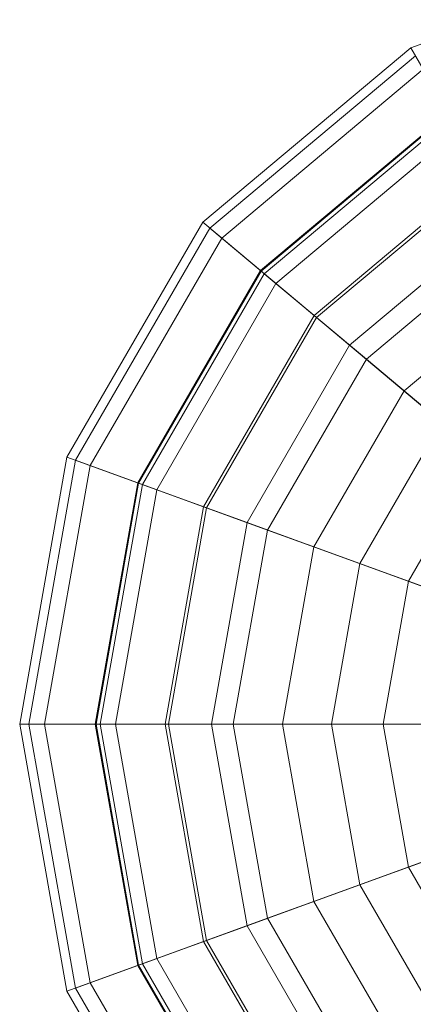
# Model space of a CAD drawing. Units: inches. Extents: x 375 to 1122, y 27 to 1069.
# Tile 31 of 155: x 731.708 to 732.389, y 280.756 to 282.464. Entities that reach past the tile are written whole.
import ezdxf

# ---------------------------------------------------------------- set-up
doc = ezdxf.new("R2010")
doc.units = ezdxf.units.IN
doc.layers.add('Furniture', color=30, linetype='Continuous', lineweight=18)

# ---------------------------------------------------------------- blocks, each defined once
blk = doc.blocks.new('A$C403C54AD')
for points in [[(1.593116, 1.197037, -0.04658), (1.626464, 1.202917, -0.043501), (1.626464, 1.202917, -0.043501), (1.597139, 1.185986, -0.04658)], [(1.597139, 1.185986, -0.04658), (1.626464, 1.202917, -0.043501), (1.626464, 1.202917, -0.043501), (1.604698, 1.176977, -0.04658)], [(1.604698, 1.176977, -0.04658), (1.626464, 1.202917, -0.043501), (1.626464, 1.202917, -0.043501), (1.614883, 1.171097, -0.04658)], [(1.614883, 1.171097, -0.04658), (1.626464, 1.202917, -0.043501), (1.626464, 1.202917, -0.043501), (1.626464, 1.169055, -0.04658)], [(1.65579, 1.185986, -0.04658), (1.626464, 1.202917, -0.043501), (1.626464, 1.202917, -0.043501), (1.659812, 1.197037, -0.04658)], [(1.64823, 1.176977, -0.04658), (1.626464, 1.202917, -0.043501), (1.626464, 1.202917, -0.043501), (1.65579, 1.185986, -0.04658)], [(1.638046, 1.171097, -0.04658), (1.626464, 1.202917, -0.043501), (1.626464, 1.202917, -0.043501), (1.64823, 1.176977, -0.04658)], [(1.626464, 1.169055, -0.04658), (1.626464, 1.202917, -0.043501), (1.626464, 1.202917, -0.043501), (1.638046, 1.171097, -0.04658)], [(1.596333, 1.197604, -0.043349), (1.593116, 1.197037, -0.04658), (1.597139, 1.185986, -0.04658), (1.599967, 1.187619, -0.043349)], [(1.620741, 1.196096, 0.042248), (1.614812, 1.189031, 0.048884), (1.620264, 1.185883, 0.048884), (1.623419, 1.19455, 0.042248)], [(1.62951, 1.19455, 0.042248), (1.632664, 1.185883, 0.048884), (1.638116, 1.189031, 0.048884), (1.632188, 1.196096, 0.042248)], [(1.614154, 1.19581, -0.040074), (1.599967, 1.187619, -0.043349), (1.606797, 1.179479, -0.043349), (1.617327, 1.192029, -0.040074)], [(1.635601, 1.192029, -0.040074), (1.646131, 1.179479, -0.043349), (1.652961, 1.187619, -0.043349), (1.638774, 1.19581, -0.040074)], [(1.613379, 1.187323, 0.046697), (1.61996, 1.195166, 0.03933), (1.623003, 1.193409, 0.03933), (1.619501, 1.183788, 0.046697)], [(1.633427, 1.183788, 0.046697), (1.629925, 1.193409, 0.03933), (1.632968, 1.195166, 0.03933), (1.63955, 1.187323, 0.046697)], [(1.623419, 1.19455, 0.042248), (1.620264, 1.185883, 0.048884), (1.626464, 1.18479, 0.048884), (1.626464, 1.194013, 0.042248)], [(1.626464, 1.194013, 0.042248), (1.626464, 1.18479, 0.048884), (1.632664, 1.185883, 0.048884), (1.62951, 1.19455, 0.042248)], [(1.610766, 1.193854, 0.048884), (1.605149, 1.190611, 0.058276), (1.610643, 1.184063, 0.058276), (1.614812, 1.189031, 0.048884)], [(1.638116, 1.189031, 0.048884), (1.642285, 1.184063, 0.058276), (1.64778, 1.190611, 0.058276), (1.642163, 1.193854, 0.048884)], [(1.619501, 1.183788, 0.046697), (1.623003, 1.193409, 0.03933), (1.626464, 1.192799, 0.03933), (1.626464, 1.18256, 0.046697)], [(1.626464, 1.18256, 0.046697), (1.626464, 1.192799, 0.03933), (1.629925, 1.193409, 0.03933), (1.633427, 1.183788, 0.046697)], [(1.602714, 1.189206, 0.056929), (1.608834, 1.192739, 0.046697), (1.613379, 1.187323, 0.046697), (1.608836, 1.18191, 0.056929)], [(1.617327, 1.192029, -0.040074), (1.606797, 1.179479, -0.043349), (1.616, 1.174166, -0.043349), (1.621603, 1.18956, -0.040074)], [(1.631326, 1.18956, -0.040074), (1.636929, 1.174166, -0.043349), (1.646131, 1.179479, -0.043349), (1.635601, 1.192029, -0.040074)], [(1.602589, 1.189133, 0.115599), (1.606995, 1.191677, 0.12581), (1.612014, 1.185696, 0.12581), (1.608743, 1.181798, 0.115599)], [(1.606995, 1.191677, 0.12581), (1.604329, 1.190138, 0.12581), (1.610035, 1.183338, 0.12581), (1.612014, 1.185696, 0.12581)], [(1.605149, 1.190611, 0.058276), (1.600725, 1.188057, 0.075423), (1.60736, 1.18015, 0.075423), (1.610643, 1.184063, 0.058276)], [(1.604329, 1.190138, 0.12581), (1.600002, 1.187639, 0.116404), (1.606823, 1.17951, 0.116404), (1.610035, 1.183338, 0.12581)], [(1.621603, 1.18956, -0.040074), (1.616, 1.174166, -0.043349), (1.626464, 1.172321, -0.043349), (1.626464, 1.188703, -0.040074)], [(1.626464, 1.188703, -0.040074), (1.626464, 1.172321, -0.043349), (1.636929, 1.174166, -0.043349), (1.631326, 1.18956, -0.040074)], [(1.598069, 1.186523, 0.074938), (1.602714, 1.189206, 0.056929), (1.608836, 1.18191, 0.056929), (1.605388, 1.1778, 0.074938)], [(1.600155, 1.187728, 0.102963), (1.602589, 1.189133, 0.115599), (1.608743, 1.181798, 0.115599), (1.606937, 1.179646, 0.102963)], [(1.614812, 1.189031, 0.048884), (1.610643, 1.184063, 0.058276), (1.618046, 1.179789, 0.058276), (1.620264, 1.185883, 0.048884)], [(1.632664, 1.185883, 0.048884), (1.634882, 1.179789, 0.058276), (1.642285, 1.184063, 0.058276), (1.638116, 1.189031, 0.048884)], [(1.600725, 1.188057, 0.075423), (1.600155, 1.187728, 0.102963), (1.606937, 1.179646, 0.102963), (1.60736, 1.18015, 0.075423)], [(1.599967, 1.187619, -0.043349), (1.597139, 1.185986, -0.04658), (1.604698, 1.176977, -0.04658), (1.606797, 1.179479, -0.043349)], [(1.600002, 1.187639, 0.116404), (1.597484, 1.186186, 0.10318), (1.604954, 1.177283, 0.10318), (1.606823, 1.17951, 0.116404)], [(1.608836, 1.18191, 0.056929), (1.613379, 1.187323, 0.046697), (1.619501, 1.183788, 0.046697), (1.617085, 1.177147, 0.056929)], [(1.635844, 1.177147, 0.056929), (1.633427, 1.183788, 0.046697), (1.63955, 1.187323, 0.046697), (1.644092, 1.18191, 0.056929)], [(1.597484, 1.186186, 0.10318), (1.598069, 1.186523, 0.074938), (1.605388, 1.1778, 0.074938), (1.604954, 1.177283, 0.10318)], [(1.608743, 1.181798, 0.115599), (1.612014, 1.185696, 0.12581), (1.618775, 1.181792, 0.12581), (1.617035, 1.177011, 0.115599)], [(1.612014, 1.185696, 0.12581), (1.610035, 1.183338, 0.12581), (1.617722, 1.178899, 0.12581), (1.618775, 1.181792, 0.12581)], [(1.620264, 1.185883, 0.048884), (1.618046, 1.179789, 0.058276), (1.626464, 1.178304, 0.058276), (1.626464, 1.18479, 0.048884)], [(1.626464, 1.18479, 0.048884), (1.626464, 1.178304, 0.058276), (1.634882, 1.179789, 0.058276), (1.632664, 1.185883, 0.048884)], [(1.634153, 1.181792, 0.12581), (1.635206, 1.178899, 0.12581), (1.642894, 1.183338, 0.12581), (1.640915, 1.185696, 0.12581)], [(1.635893, 1.177011, 0.115599), (1.634153, 1.181792, 0.12581), (1.640915, 1.185696, 0.12581), (1.644185, 1.181798, 0.115599)], [(1.610643, 1.184063, 0.058276), (1.60736, 1.18015, 0.075423), (1.616299, 1.174989, 0.075423), (1.618046, 1.179789, 0.058276)], [(1.634882, 1.179789, 0.058276), (1.636629, 1.174989, 0.075423), (1.645568, 1.18015, 0.075423), (1.642285, 1.184063, 0.058276)], [(1.617085, 1.177147, 0.056929), (1.619501, 1.183788, 0.046697), (1.626464, 1.18256, 0.046697), (1.626464, 1.175494, 0.056929)], [(1.626464, 1.175494, 0.056929), (1.626464, 1.18256, 0.046697), (1.633427, 1.183788, 0.046697), (1.635844, 1.177147, 0.056929)], [(1.610035, 1.183338, 0.12581), (1.606823, 1.17951, 0.116404), (1.616013, 1.174204, 0.116404), (1.617722, 1.178899, 0.12581)], [(1.635206, 1.178899, 0.12581), (1.636915, 1.174204, 0.116404), (1.646105, 1.17951, 0.116404), (1.642894, 1.183338, 0.12581)], [(1.605388, 1.1778, 0.074938), (1.608836, 1.18191, 0.056929), (1.617085, 1.177147, 0.056929), (1.61525, 1.172106, 0.074938)], [(1.606937, 1.179646, 0.102963), (1.608743, 1.181798, 0.115599), (1.617035, 1.177011, 0.115599), (1.616074, 1.174371, 0.102963)], [(1.617035, 1.177011, 0.115599), (1.618775, 1.181792, 0.12581), (1.626464, 1.180436, 0.12581), (1.626464, 1.175348, 0.115599)], [(1.618775, 1.181792, 0.12581), (1.617722, 1.178899, 0.12581), (1.626464, 1.177358, 0.12581), (1.626464, 1.180436, 0.12581)], [(1.626464, 1.180436, 0.12581), (1.626464, 1.177358, 0.12581), (1.635206, 1.178899, 0.12581), (1.634153, 1.181792, 0.12581)], [(1.626464, 1.175348, 0.115599), (1.626464, 1.180436, 0.12581), (1.634153, 1.181792, 0.12581), (1.635893, 1.177011, 0.115599)], [(1.637678, 1.172106, 0.074938), (1.635844, 1.177147, 0.056929), (1.644092, 1.18191, 0.056929), (1.64754, 1.1778, 0.074938)], [(1.636854, 1.174371, 0.102963), (1.635893, 1.177011, 0.115599), (1.644185, 1.181798, 0.115599), (1.645991, 1.179646, 0.102963)], [(1.60736, 1.18015, 0.075423), (1.606937, 1.179646, 0.102963), (1.616074, 1.174371, 0.102963), (1.616299, 1.174989, 0.075423)], [(1.636629, 1.174989, 0.075423), (1.636854, 1.174371, 0.102963), (1.645991, 1.179646, 0.102963), (1.645568, 1.18015, 0.075423)], [(1.618046, 1.179789, 0.058276), (1.616299, 1.174989, 0.075423), (1.626464, 1.173197, 0.075423), (1.626464, 1.178304, 0.058276)], [(1.626464, 1.178304, 0.058276), (1.626464, 1.173197, 0.075423), (1.636629, 1.174989, 0.075423), (1.634882, 1.179789, 0.058276)], [(1.606797, 1.179479, -0.043349), (1.604698, 1.176977, -0.04658), (1.614883, 1.171097, -0.04658), (1.616, 1.174166, -0.043349)], [(1.606823, 1.17951, 0.116404), (1.604954, 1.177283, 0.10318), (1.615019, 1.171472, 0.10318), (1.616013, 1.174204, 0.116404)], [(1.636915, 1.174204, 0.116404), (1.637909, 1.171472, 0.10318), (1.647974, 1.177283, 0.10318), (1.646105, 1.17951, 0.116404)], [(1.636929, 1.174166, -0.043349), (1.638046, 1.171097, -0.04658), (1.64823, 1.176977, -0.04658), (1.646131, 1.179479, -0.043349)], [(1.617722, 1.178899, 0.12581), (1.616013, 1.174204, 0.116404), (1.626464, 1.172361, 0.116404), (1.626464, 1.177358, 0.12581)], [(1.626464, 1.177358, 0.12581), (1.626464, 1.172361, 0.116404), (1.636915, 1.174204, 0.116404), (1.635206, 1.178899, 0.12581)], [(1.604954, 1.177283, 0.10318), (1.605388, 1.1778, 0.074938), (1.61525, 1.172106, 0.074938), (1.615019, 1.171472, 0.10318)], [(1.637909, 1.171472, 0.10318), (1.637678, 1.172106, 0.074938), (1.64754, 1.1778, 0.074938), (1.647974, 1.177283, 0.10318)], [(1.61525, 1.172106, 0.074938), (1.617085, 1.177147, 0.056929), (1.626464, 1.175494, 0.056929), (1.626464, 1.170129, 0.074938)], [(1.626464, 1.170129, 0.074938), (1.626464, 1.175494, 0.056929), (1.635844, 1.177147, 0.056929), (1.637678, 1.172106, 0.074938)], [(1.616074, 1.174371, 0.102963), (1.617035, 1.177011, 0.115599), (1.626464, 1.175348, 0.115599), (1.626464, 1.172539, 0.102963)], [(1.626464, 1.172539, 0.102963), (1.626464, 1.175348, 0.115599), (1.635893, 1.177011, 0.115599), (1.636854, 1.174371, 0.102963)], [(1.616299, 1.174989, 0.075423), (1.616074, 1.174371, 0.102963), (1.626464, 1.172539, 0.102963), (1.626464, 1.173197, 0.075423)], [(1.626464, 1.173197, 0.075423), (1.626464, 1.172539, 0.102963), (1.636854, 1.174371, 0.102963), (1.636629, 1.174989, 0.075423)], [(1.616, 1.174166, -0.043349), (1.614883, 1.171097, -0.04658), (1.626464, 1.169055, -0.04658), (1.626464, 1.172321, -0.043349)], [(1.616013, 1.174204, 0.116404), (1.615019, 1.171472, 0.10318), (1.626464, 1.169454, 0.10318), (1.626464, 1.172361, 0.116404)], [(1.626464, 1.172361, 0.116404), (1.626464, 1.169454, 0.10318), (1.637909, 1.171472, 0.10318), (1.636915, 1.174204, 0.116404)], [(1.626464, 1.172321, -0.043349), (1.626464, 1.169055, -0.04658), (1.638046, 1.171097, -0.04658), (1.636929, 1.174166, -0.043349)], [(1.615019, 1.171472, 0.10318), (1.61525, 1.172106, 0.074938), (1.626464, 1.170129, 0.074938), (1.626464, 1.169454, 0.10318)], [(1.626464, 1.169454, 0.10318), (1.626464, 1.170129, 0.074938), (1.637678, 1.172106, 0.074938), (1.637909, 1.171472, 0.10318)]]:
    blk.add_3dface(points)

msp = doc.modelspace()

# ---------------------------------------------------------------- block references
at = {"layer": 'Furniture', "xscale": 39.9918517141215, "yscale": 39.9918517141215, "zscale": 39.9918517141215, "rotation": 270}
msp.add_blockref('A$C403C54AD', (684.9549, 346.2875, 0.024), dxfattribs=at)

doc.saveas('drawing.dxf')
